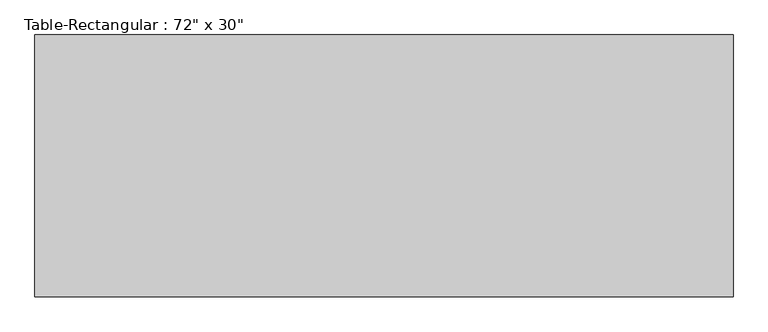
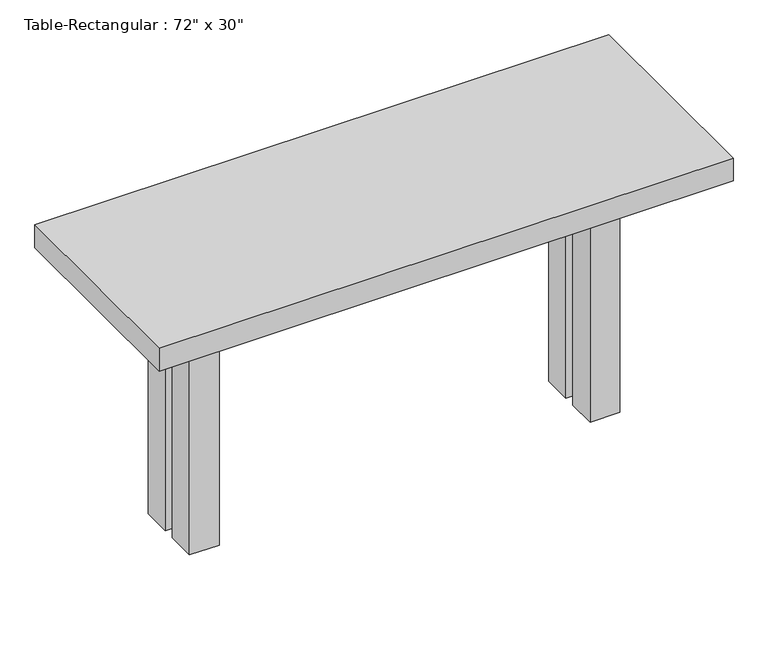
"""IFC4 building model written with IfcOpenShell, lengths in millimetres: furniture geometry."""

from ifc_helpers import new_model, si_unit, frame, origin, origin_with_axes, place, context, project, spatial, polyline, outline, extrude, source, transform, mapped, element, save


def furniture_c21ab0ed(model_context):
    return source(origin(), model_context, "Body", "SweptSolid", [
        extrude(outline(polyline([(393.7, 38.1), (393.7, 12.7), (-393.7, 12.7), (-393.7, 38.1), (393.7, 38.1)])), frame((0.0, 0.0, 457.2), z_axis=(0.0, 0.0, 1.0), x_axis=(1.0, 0.0, 0.0)), (0.0, 0.0, 1.0), 101.6),
        extrude(outline(polyline([(393.7, -38.1), (-393.7, -38.1), (-393.7, -12.7), (393.7, -12.7), (393.7, -38.1)])), frame((0.0, 0.0, 457.2), z_axis=(0.0, 0.0, 1.0), x_axis=(1.0, 0.0, 0.0)), (0.0, 0.0, 1.0), 101.6),
        extrude(outline(polyline([(-406.4, -12.7), (-431.8, -12.7), (-431.8, 12.7), (-406.4, 12.7), (-406.4, -12.7)])), frame((0.0, 0.0, 457.2), z_axis=(0.0, 0.0, 1.0), x_axis=(1.0, 0.0, 0.0)), (0.0, 0.0, 1.0), 101.6),
        extrude(outline(polyline([(406.4, -12.7), (406.4, 12.7), (431.8, 12.7), (431.8, -12.7), (406.4, -12.7)])), frame((0.0, 0.0, 457.2), z_axis=(0.0, 0.0, 1.0), x_axis=(1.0, 0.0, 0.0)), (0.0, 0.0, 1.0), 101.6),
        extrude(outline(polyline([(609.6, 228.6), (609.6, -228.6), (-609.6, -228.6), (-609.6, 228.6), (609.6, 228.6)])), frame((0.0, 0.0, 558.8), z_axis=(0.0, 0.0, 1.0), x_axis=(1.0, 0.0, 0.0)), (0.0, 0.0, 1.0), 50.8),
        extrude(outline(polyline([(-393.7, 76.2), (-393.7, 12.7), (-457.2, 12.7), (-457.2, 76.2), (-393.7, 76.2)])), origin_with_axes(), (0.0, 0.0, 1.0), 558.8),
        extrude(outline(polyline([(393.7, 76.2), (457.2, 76.2), (457.2, 12.7), (393.7, 12.7), (393.7, 76.2)])), origin_with_axes(), (0.0, 0.0, 1.0), 558.8),
        extrude(outline(polyline([(-393.7, -76.2), (-457.2, -76.2), (-457.2, -12.7), (-393.7, -12.7), (-393.7, -76.2)])), origin_with_axes(), (0.0, 0.0, 1.0), 558.8),
        extrude(outline(polyline([(393.7, -76.2), (393.7, -12.7), (457.2, -12.7), (457.2, -76.2), (393.7, -76.2)])), origin_with_axes(), (0.0, 0.0, 1.0), 558.8),
    ])


if __name__ == "__main__":
    model = new_model("IFC4")
    model_context = context("Model", 3, world=origin())
    ifc_project = project(units=[si_unit("LENGTHUNIT", "METRE", prefix="MILLI")], contexts=[model_context])
    site = spatial("IfcSite", under=ifc_project)
    building = spatial("IfcBuilding", under=site)
    placement = place(None, origin())
    furniture_shape = furniture_c21ab0ed(model_context)
    element("IfcFurniture", 1, ObjectType="Table-Rectangular : 72\" x 30\"", at=placement, inside=building, context=model_context, shape_type="MappedRepresentation", body=[
        mapped(furniture_shape, transform((0.0, 0.0, 0.0), x_axis=(1.0, 0.0, 0.0), y_axis=(0.0, 1.0, 0.0), z_axis=(0.0, 0.0, 1.0))),
    ])
    save(model, "model.ifc")

# Revit data of these elements
# Type "Table-Rectangular : 72\" x 30\""
#   Assembly Code = "E2020200"
#   Height = 2' - 0"
#   Length = 4' - 0"
#   Width = 1' - 6"
#   Base Material = Birch
#   Top Material = Birch
#   Default Elevation = 0
# Element 1 (IfcFurniture, "Table-Rectangular : 72\" x 30\"")
#   Materials on its faces: "Birch"
# Materials
#   "Birch": class "Wood", colour RGB 224 178 126, transparency 0, Description = "Betula Alleghaniensis", Cost = 0
